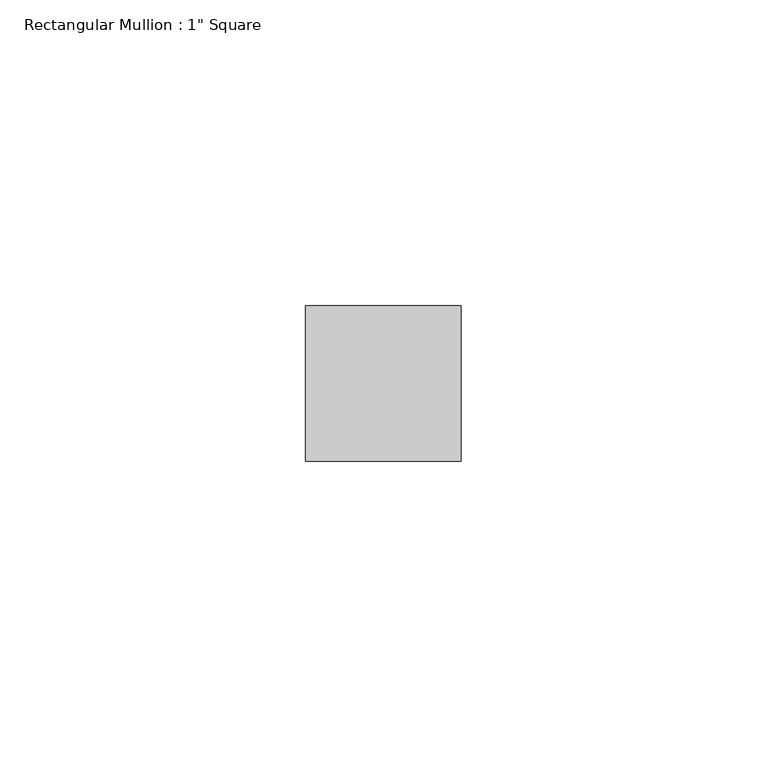
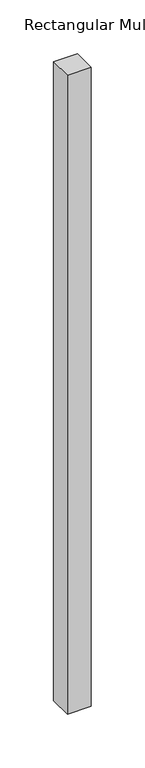
"""IFC4 building model written with IfcOpenShell, lengths in millimetres: member geometry."""

from ifc_helpers import new_model, si_unit, frame, origin, place, context, project, spatial, polyline, outline, extrude, source, transform, mapped, element, save


def member_f362a377(model_context):
    return source(origin(), model_context, "Body", "SweptSolid", [
        extrude(outline(polyline([(0.0, 12.7), (0.0, -12.7), (-25.4, -12.7), (-25.4, 12.7), (0.0, 12.7)])), frame((0.0, 0.0, -723.9), z_axis=(0.0, 0.0, 1.0), x_axis=(1.0, 0.0, 0.0)), (0.0, 0.0, 1.0), 723.9),
    ])


if __name__ == "__main__":
    model = new_model("IFC4")
    model_context = context("Model", 3, world=origin())
    ifc_project = project(units=[si_unit("LENGTHUNIT", "METRE", prefix="MILLI")], contexts=[model_context])
    site = spatial("IfcSite", under=ifc_project)
    building = spatial("IfcBuilding", under=site)
    placement = place(None, origin())
    member_shape = member_f362a377(model_context)
    element("IfcMember", 1, ObjectType="Rectangular Mullion : 1\" Square", at=placement, inside=building, context=model_context, shape_type="MappedRepresentation", body=[
        mapped(member_shape, transform((0.0, 0.0, 0.0), x_axis=(1.0, 0.0, 0.0), y_axis=(0.0, 1.0, 0.0), z_axis=(0.0, 0.0, 1.0))),
    ])
    save(model, "model.ifc")

# Revit data of these elements
# Type "Rectangular Mullion : 1\" Square"
#   built-in parameter 1007304 = 0.0833333 (stored number, unit not read)
#   built-in parameter 1007301 = 0.0416667 (stored number, unit not read)
#   built-in parameter 1007300 = 0.0416667 (stored number, unit not read)
